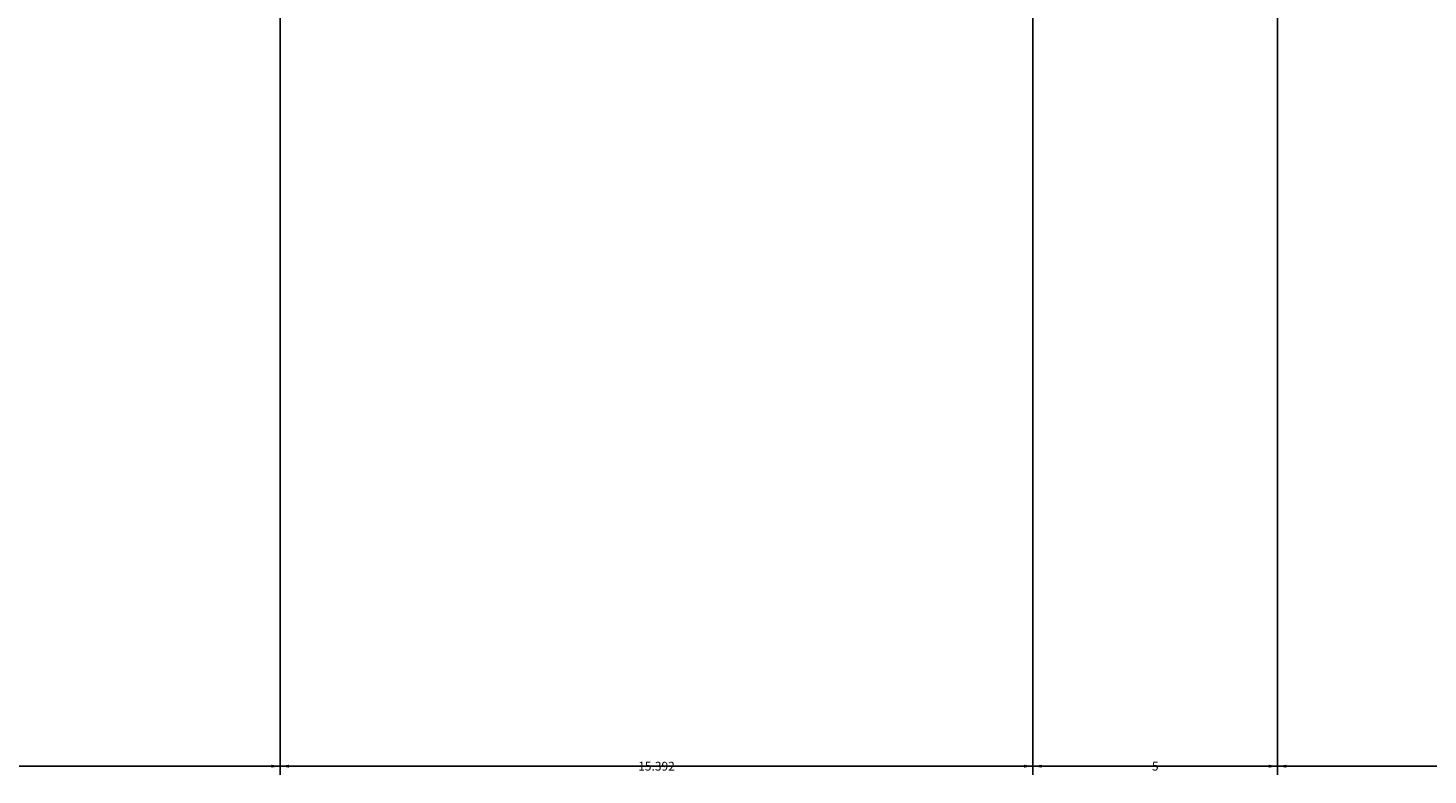
# Model space of a CAD drawing. Units: inches. Extents: x -6 to 289, y -8 to 323.
# Tile 3 of 107: x 19 to 48, y -8 to 7. Entities that reach past the tile are written whole.
import ezdxf

# ---------------------------------------------------------------- set-up
doc = ezdxf.new("R2010")
doc.units = ezdxf.units.IN
doc.header["$MEASUREMENT"] = 0
doc.layers.add('A-ANNO-DIMS', color=2, linetype='Continuous', lineweight=18)
doc.styles.get("Standard").update_dxf_attribs({"font": 'arial.ttf'})
doc.dimstyles.get("Standard").update_dxf_attribs({"dimtxt": 0.18, "dimasz": 0.18, "dimexe": 0.18, "dimexo": 0.0625, "dimgap": 0.09, "dimtad": 0, "dimtih": 1, "dimtoh": 1, "dimdec": 4, "dimzin": 0, "dimdsep": 46, "dimtxsty": 'Standard', "dimcen": 0.09, "dimadec": 0, "dimazin": 0, "dimtfac": 1, "dimtdec": 4, "dimtofl": 0, "dimtmove": 0, "dimatfit": 3, "dimfxl": 1, "dimtolj": 1, "dimtzin": 0, "dimarcsym": 0})

# ---------------------------------------------------------------- blocks, each defined once
blk = doc.blocks.new('*D16')
at = {"layer": 'A-ANNO-DIMS', "color": 0, "lineweight": -2, "transparency": 16777216}
for p, q in [((9.943, 68.37), (9.943, -8.391)), ((272.973, 68.37), (272.973, -8.391)), ((10.123, -8.211), (140.993, -8.211)), ((272.793, -8.211), (141.923, -8.211))]:
    blk.add_line(p, q, dxfattribs=at)
at = {"layer": 'A-ANNO-DIMS', "color": 0, "transparency": 16777216}
for points in [[(10.123, -8.181), (10.123, -8.241), (9.943, -8.211)], [(272.793, -8.181), (272.793, -8.241), (272.973, -8.211)]]:
    blk.add_solid(points, dxfattribs=at)
at = {"layer": 'Defpoints', "color": 0, "transparency": 16777216}
for p in [(9.943, 68.432), (272.973, 68.432), (272.973, -8.211)]:
    blk.add_point(p, dxfattribs=at)
at = {"layer": 'A-ANNO-DIMS', "color": 0, "transparency": 16777216, "insert": (141.458, -8.211), "char_height": 0.18, "attachment_point": 5}
blk.add_mtext('\\A1;263.03', dxfattribs=at)
blk = doc.blocks.new('*D50')
at = {"layer": 'A-ANNO-DIMS', "color": 0, "lineweight": -2, "transparency": 16777216}
for p, q in [((11.969, 7.226), (11.969, -8.391)), ((24.317, 7.226), (24.317, -8.391)), ((12.149, -8.211), (17.688, -8.211)), ((24.137, -8.211), (18.598, -8.211))]:
    blk.add_line(p, q, dxfattribs=at)
at = {"layer": 'A-ANNO-DIMS', "color": 0, "transparency": 16777216}
for points in [[(12.149, -8.181), (12.149, -8.241), (11.969, -8.211)], [(24.137, -8.181), (24.137, -8.241), (24.317, -8.211)]]:
    blk.add_solid(points, dxfattribs=at)
at = {"layer": 'Defpoints', "color": 0, "transparency": 16777216}
for p in [(11.969, 7.289), (24.317, 7.289), (24.317, -8.211)]:
    blk.add_point(p, dxfattribs=at)
at = {"layer": 'A-ANNO-DIMS', "color": 0, "transparency": 16777216, "insert": (18.143, -8.211), "char_height": 0.18, "attachment_point": 5}
blk.add_mtext('\\A1;12.348', dxfattribs=at)
blk = doc.blocks.new('*D51')
at = {"layer": 'A-ANNO-DIMS', "color": 0, "lineweight": -2, "transparency": 16777216}
for p, q in [((39.709, 16.629), (39.709, -8.391)), ((24.317, 7.226), (24.317, -8.391)), ((24.497, -8.211), (31.559, -8.211)), ((39.529, -8.211), (32.467, -8.211))]:
    blk.add_line(p, q, dxfattribs=at)
at = {"layer": 'A-ANNO-DIMS', "color": 0, "transparency": 16777216}
for points in [[(24.497, -8.181), (24.497, -8.241), (24.317, -8.211)], [(39.529, -8.181), (39.529, -8.241), (39.709, -8.211)]]:
    blk.add_solid(points, dxfattribs=at)
at = {"layer": 'Defpoints', "color": 0, "transparency": 16777216}
for p in [(39.709, 16.692), (24.317, 7.289), (39.709, -8.211)]:
    blk.add_point(p, dxfattribs=at)
at = {"layer": 'A-ANNO-DIMS', "color": 0, "transparency": 16777216, "insert": (32.013, -8.211), "char_height": 0.18, "attachment_point": 5}
blk.add_mtext('\\A1;15.392', dxfattribs=at)
blk = doc.blocks.new('*D52')
at = {"layer": 'A-ANNO-DIMS', "color": 0, "lineweight": -2, "transparency": 16777216}
for p, q in [((44.709, 21.629), (44.709, -8.391)), ((39.709, 16.629), (39.709, -8.391)), ((39.889, -8.211), (42.059, -8.211)), ((44.529, -8.211), (42.359, -8.211))]:
    blk.add_line(p, q, dxfattribs=at)
at = {"layer": 'A-ANNO-DIMS', "color": 0, "transparency": 16777216}
for points in [[(39.889, -8.181), (39.889, -8.241), (39.709, -8.211)], [(44.529, -8.181), (44.529, -8.241), (44.709, -8.211)]]:
    blk.add_solid(points, dxfattribs=at)
at = {"layer": 'Defpoints', "color": 0, "transparency": 16777216}
for p in [(44.709, 21.692), (39.709, 16.692), (44.709, -8.211)]:
    blk.add_point(p, dxfattribs=at)
at = {"layer": 'A-ANNO-DIMS', "color": 0, "transparency": 16777216, "insert": (42.209, -8.211), "char_height": 0.18, "attachment_point": 5}
blk.add_mtext('\\A1;5', dxfattribs=at)
blk = doc.blocks.new('*D53')
at = {"layer": 'A-ANNO-DIMS', "color": 0, "lineweight": -2, "transparency": 16777216}
for p, q in [((44.709, 21.629), (44.709, -8.391)), ((87.562, 21.629), (87.562, -8.391)), ((44.889, -8.211), (65.738, -8.211)), ((87.382, -8.211), (66.534, -8.211))]:
    blk.add_line(p, q, dxfattribs=at)
at = {"layer": 'A-ANNO-DIMS', "color": 0, "transparency": 16777216}
for points in [[(44.889, -8.181), (44.889, -8.241), (44.709, -8.211)], [(87.382, -8.181), (87.382, -8.241), (87.562, -8.211)]]:
    blk.add_solid(points, dxfattribs=at)
at = {"layer": 'Defpoints', "color": 0, "transparency": 16777216}
for p in [(44.709, 21.692), (87.562, 21.692), (87.562, -8.211)]:
    blk.add_point(p, dxfattribs=at)
at = {"layer": 'A-ANNO-DIMS', "color": 0, "transparency": 16777216, "insert": (66.136, -8.211), "char_height": 0.18, "attachment_point": 5}
blk.add_mtext('\\A1;42.85', dxfattribs=at)

msp = doc.modelspace()

# ---------------------------------------------------------------- dimensions: what is measured, and where the dimension line sits
at = {"layer": 'A-ANNO-DIMS'}
for base, p1, p2, override, picture, middle in [((272.9733, -8.2112), (9.943, 68.4322), (272.9733, 68.4322), {"dimdec": 2, "dimlfac": 1, "dimrnd": 0, "dimzin": 0, "dimdsep": 46, "dimlunit": 2}, '*D16', (141.4581, -8.2112)), ((44.709, -8.2112), (39.709, 16.6917), (44.709, 21.6917), {"dimdec": 0, "dimlfac": 1, "dimrnd": 0, "dimzin": 0, "dimdsep": 46, "dimlunit": 2}, '*D52', (42.209, -8.2112)), ((87.5623, -8.2112), (44.709, 21.6917), (87.5623, 21.6917), {"dimdec": 2, "dimlfac": 1, "dimrnd": 0, "dimzin": 0, "dimdsep": 46, "dimlunit": 2}, '*D53', (66.1357, -8.2112)), ((39.709, -8.2112), (24.317, 7.2888), (39.709, 16.6917), {"dimdec": 3, "dimlfac": 1, "dimrnd": 0, "dimzin": 0, "dimdsep": 46, "dimlunit": 2}, '*D51', (32.013, -8.2112)), ((24.317, -8.2112), (11.9692, 7.2888), (24.317, 7.2888), {"dimdec": 3, "dimlfac": 1, "dimrnd": 0, "dimzin": 0, "dimdsep": 46, "dimlunit": 2}, '*D50', (18.1431, -8.2112))]:
    dim = msp.add_linear_dim(base=base, p1=p1, p2=p2, dimstyle='Standard', override=override, dxfattribs=at)
    dim.commit()
    dim.dimension.update_dxf_attribs({"geometry": picture, "text_midpoint": middle})

doc.saveas('drawing.dxf')
